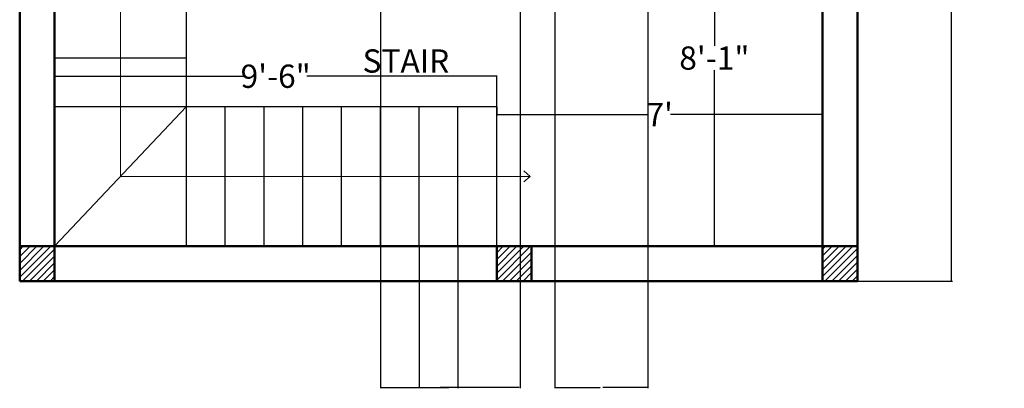
# Model space of a CAD drawing. Units: inches. Extents: x 0 to 281, y -535 to 46.
# Tile 1 of 22: x 27 to 281, y -535 to -440. Entities that reach past the tile are written whole.
import ezdxf

# ---------------------------------------------------------------- set-up
doc = ezdxf.new("R2010")
doc.units = ezdxf.units.IN
doc.header["$MEASUREMENT"] = 0
for name, color, linetype, lineweight in [('A-ANNO-DIMS', 2, 'Continuous', 18), ('A-ANNO-SYMB', 2, 'Continuous', 18), ('A-AREA-IDEN', 7, 'Continuous', 25), ('A-COLS', 7, 'Continuous', 50), ('A-COLS-PATT', 152, 'Continuous', 13), ('A-FLOR-STRS', 7, 'Continuous', 25), ('A-WALL', 7, 'Continuous', 50)]:
    doc.layers.add(name, color=color, linetype=linetype, lineweight=lineweight)
doc.styles.get("Standard").update_dxf_attribs({"font": 'arial.ttf'})
doc.dimstyles.get("Standard").update_dxf_attribs({"dimtxt": 0.18, "dimasz": 0.18, "dimexe": 0.18, "dimexo": 0.0625, "dimgap": 0.09, "dimtad": 0, "dimtih": 1, "dimtoh": 1, "dimdec": 0, "dimzin": 0, "dimdsep": 46, "dimlunit": 3, "dimtxsty": 'Standard', "dimcen": 0.09, "dimadec": 0, "dimazin": 0, "dimtfac": 1, "dimtdec": 0, "dimtofl": 0, "dimtmove": 0, "dimatfit": 3, "dimfxl": 1, "dimtolj": 1, "dimtzin": 0, "dimarcsym": 0})

# ---------------------------------------------------------------- blocks, each defined once
blk = doc.blocks.new('*D13')
at = {"layer": 'A-ANNO-DIMS', "color": 0, "lineweight": -2, "transparency": 16777216}
for p, q in [((206.57, -401.59), (206.57, -446.76)), ((206.63, -401.41), (206.75, -401.41)), ((206.57, -498.23), (206.57, -453.06)), ((206.63, -498.41), (206.75, -498.41))]:
    blk.add_line(p, q, dxfattribs=at)
at = {"layer": 'A-ANNO-DIMS', "color": 0, "transparency": 16777216}
for points in [[(206.54, -401.59), (206.6, -401.59), (206.57, -401.41)], [(206.54, -498.23), (206.6, -498.23), (206.57, -498.41)]]:
    blk.add_solid(points, dxfattribs=at)
at = {"layer": 'Defpoints', "color": 0, "transparency": 16777216}
for p in [(206.57, -401.41), (206.57, -498.41), (206.57, -498.41)]:
    blk.add_point(p, dxfattribs=at)
at = {"layer": 'A-ANNO-DIMS', "color": 0, "transparency": 16777216, "insert": (206.57, -449.91), "char_height": 6, "attachment_point": 5}
blk.add_mtext('\\A1;8\'-1"', dxfattribs=at)
blk = doc.blocks.new('*D14')
at = {"layer": 'A-ANNO-DIMS', "color": 0, "lineweight": -2, "transparency": 16777216}
for p, q in [((150.46, -462.47), (150.46, -464.67)), ((150.64, -464.49), (189.63, -464.49)), ((234.28, -464.49), (195.28, -464.49)), ((234.46, -462.47), (234.46, -464.67))]:
    blk.add_line(p, q, dxfattribs=at)
at = {"layer": 'A-ANNO-DIMS', "color": 0, "transparency": 16777216}
for points in [[(150.64, -464.46), (150.64, -464.52), (150.46, -464.49)], [(234.28, -464.46), (234.28, -464.52), (234.46, -464.49)]]:
    blk.add_solid(points, dxfattribs=at)
at = {"layer": 'Defpoints', "color": 0, "transparency": 16777216}
for p in [(150.46, -462.41), (234.46, -462.41), (234.46, -464.49)]:
    blk.add_point(p, dxfattribs=at)
at = {"layer": 'A-ANNO-DIMS', "color": 0, "transparency": 16777216, "insert": (192.46, -464.49), "char_height": 6, "attachment_point": 5}
blk.add_mtext("\\A1;7'", dxfattribs=at)
blk = doc.blocks.new('*D16')
at = {"layer": 'A-ANNO-DIMS', "color": 0, "lineweight": -2, "transparency": 16777216}
for p, q in [((36.46, -462.35), (36.46, -454.41)), ((150.46, -462.35), (150.46, -454.41)), ((36.64, -454.59), (85.39, -454.59)), ((150.28, -454.59), (101.52, -454.59))]:
    blk.add_line(p, q, dxfattribs=at)
at = {"layer": 'A-ANNO-DIMS', "color": 0, "transparency": 16777216}
for points in [[(36.64, -454.56), (36.64, -454.62), (36.46, -454.59)], [(150.28, -454.56), (150.28, -454.62), (150.46, -454.59)]]:
    blk.add_solid(points, dxfattribs=at)
at = {"layer": 'Defpoints', "color": 0, "transparency": 16777216}
for p in [(36.46, -454.59), (36.46, -462.41), (150.46, -462.41)]:
    blk.add_point(p, dxfattribs=at)
at = {"layer": 'A-ANNO-DIMS', "color": 0, "transparency": 16777216, "insert": (93.46, -454.59), "char_height": 6, "attachment_point": 5}
blk.add_mtext('\\A1;9\'-6"', dxfattribs=at)
blk = doc.blocks.new('*D18')
at = {"layer": 'A-ANNO-DIMS', "color": 0, "lineweight": -2, "transparency": 16777216}
for p, q in [((243.52, 18.59), (267.93, 18.59)), ((267.75, 18.41), (267.75, -241.26)), ((267.75, -507.23), (267.75, -247.57)), ((243.52, -507.41), (267.93, -507.41))]:
    blk.add_line(p, q, dxfattribs=at)
at = {"layer": 'A-ANNO-DIMS', "color": 0, "transparency": 16777216}
for points in [[(267.72, 18.41), (267.78, 18.41), (267.75, 18.59)], [(267.72, -507.23), (267.78, -507.23), (267.75, -507.41)]]:
    blk.add_solid(points, dxfattribs=at)
at = {"layer": 'Defpoints', "color": 0, "transparency": 16777216}
for p in [(243.46, 18.59), (243.46, -507.41), (267.75, -507.41)]:
    blk.add_point(p, dxfattribs=at)
at = {"layer": 'A-ANNO-DIMS', "color": 0, "transparency": 16777216, "insert": (267.75, -244.41), "char_height": 6, "attachment_point": 5}
blk.add_mtext('\\A1;43\'-10"', dxfattribs=at)
blk = doc.blocks.new('*D41')
at = {"layer": 'A-ANNO-DIMS', "color": 0, "lineweight": -2, "transparency": 16777216}
for p, q in [((120.46, -131.47), (120.46, -535.04)), ((156.46, -131.47), (156.46, -535.04)), ((120.64, -534.86), (138.13, -534.86)), ((156.28, -534.86), (138.79, -534.86))]:
    blk.add_line(p, q, dxfattribs=at)
at = {"layer": 'A-ANNO-DIMS', "color": 0, "transparency": 16777216}
for points in [[(120.64, -534.83), (120.64, -534.89), (120.46, -534.86)], [(156.28, -534.83), (156.28, -534.89), (156.46, -534.86)]]:
    blk.add_solid(points, dxfattribs=at)
at = {"layer": 'Defpoints', "color": 0, "transparency": 16777216}
for p in [(120.46, -131.41), (156.46, -131.41), (156.46, -534.86)]:
    blk.add_point(p, dxfattribs=at)
at = {"layer": 'A-ANNO-DIMS', "color": 0, "transparency": 16777216, "insert": (138.46, -534.86), "char_height": 0.18, "attachment_point": 5}
blk.add_mtext('\\A1;3\'-0"', dxfattribs=at)
blk = doc.blocks.new('*D42')
at = {"layer": 'A-ANNO-DIMS', "color": 0, "lineweight": -2, "transparency": 16777216}
for p, q in [((165.46, -131.47), (165.46, -535.04)), ((189.46, -131.47), (189.46, -535.04)), ((165.64, -534.86), (177.13, -534.86)), ((189.28, -534.86), (177.79, -534.86))]:
    blk.add_line(p, q, dxfattribs=at)
at = {"layer": 'A-ANNO-DIMS', "color": 0, "transparency": 16777216}
for points in [[(165.64, -534.83), (165.64, -534.89), (165.46, -534.86)], [(189.28, -534.83), (189.28, -534.89), (189.46, -534.86)]]:
    blk.add_solid(points, dxfattribs=at)
at = {"layer": 'Defpoints', "color": 0, "transparency": 16777216}
for p in [(165.46, -131.41), (189.46, -131.41), (189.46, -534.86)]:
    blk.add_point(p, dxfattribs=at)
at = {"layer": 'A-ANNO-DIMS', "color": 0, "transparency": 16777216, "insert": (177.46, -534.86), "char_height": 0.18, "attachment_point": 5}
blk.add_mtext('\\A1;2\'-0"', dxfattribs=at)
blk = doc.blocks.new('*D49')
at = {"layer": 'A-ANNO-DIMS', "color": 0, "lineweight": -2, "transparency": 16777216}
for p, q in [((130.46, -498.47), (130.46, -535.04)), ((140.46, -498.47), (140.46, -535.04)), ((130.64, -534.86), (135.06, -534.86)), ((140.28, -534.86), (135.86, -534.86))]:
    blk.add_line(p, q, dxfattribs=at)
at = {"layer": 'A-ANNO-DIMS', "color": 0, "transparency": 16777216}
for points in [[(130.64, -534.83), (130.64, -534.89), (130.46, -534.86)], [(140.28, -534.83), (140.28, -534.89), (140.46, -534.86)]]:
    blk.add_solid(points, dxfattribs=at)
at = {"layer": 'Defpoints', "color": 0, "transparency": 16777216}
for p in [(130.46, -498.41), (140.46, -498.41), (140.46, -534.86)]:
    blk.add_point(p, dxfattribs=at)
at = {"layer": 'A-ANNO-DIMS', "color": 0, "transparency": 16777216, "insert": (135.46, -534.86), "char_height": 0.18, "attachment_point": 5}
blk.add_mtext('\\A1;0\'-10"', dxfattribs=at)

msp = doc.modelspace()

# ---------------------------------------------------------------- hatches: boundary and pattern name
at = {"layer": 'A-COLS-PATT'}
h = msp.add_hatch(dxfattribs=at)
h.set_pattern_fill('ANSI31', color=256, scale=10)
h.paths.add_polyline_path([(36.46, 18.59), (27.46, 18.59), (27.46, 9.59), (36.46, 9.59)])
h.paths.add_polyline_path([(165.46, 18.59), (156.46, 18.59), (156.46, 9.59), (165.46, 9.59)])
h.paths.add_polyline_path([(243.46, 18.59), (234.46, 18.59), (234.46, 9.59), (243.46, 9.59)])
h.paths.add_polyline_path([(243.46, -122.41), (234.46, -122.41), (234.46, -131.41), (243.46, -131.41)])
h.paths.add_polyline_path([(36.46, -122.41), (27.46, -122.41), (27.46, -131.41), (36.46, -131.41)])
h.paths.add_polyline_path([(36.46, -498.41), (27.46, -498.41), (27.46, -507.41), (36.46, -507.41)])
h.paths.add_polyline_path([(243.46, -498.41), (234.46, -498.41), (234.46, -507.41), (243.46, -507.41)])
h.paths.add_polyline_path([(159.46, -498.41), (150.46, -498.41), (150.46, -507.41), (159.46, -507.41)])
h.paths.add_polyline_path([(36.46, -392.41), (27.46, -392.41), (27.46, -401.41), (36.46, -401.41)])
h.paths.add_polyline_path([(159.46, -392.41), (150.46, -392.41), (150.46, -401.41), (159.46, -401.41)])
h.paths.add_polyline_path([(243.46, -392.41), (234.46, -392.41), (234.46, -401.41), (243.46, -401.41)])
h.paths.add_polyline_path([(36.46, -263.41), (27.46, -263.41), (27.46, -272.41), (36.46, -272.41)])
h.paths.add_polyline_path([(243.46, -263.41), (234.46, -263.41), (234.46, -272.41), (243.46, -272.41)])

# ---------------------------------------------------------------- linework, layer by layer
at = {"layer": 'A-ANNO-SYMB'}
for p, q in [((53.46, -419.41), (53.46, -480.41)), ((159.11, -480.41), (157.42, -479)), ((53.46, -480.41), (159.11, -480.41)), ((159.11, -480.41), (157.42, -481.82))]:
    msp.add_line(p, q, dxfattribs=at)
at = {"layer": 'A-COLS'}
for p, q in [((150.46, -498.41), (150.46, -507.41)), ((159.46, -498.41), (159.46, -507.41))]:
    msp.add_line(p, q, dxfattribs=at)
at = {"layer": 'A-FLOR-STRS'}
for p, q in [((70.46, -498.41), (70.46, -401.41)), ((70.46, -449.91), (36.46, -449.91)), ((36.46, -462.41), (150.46, -462.41)), ((70.46, -462.41), (36.46, -498.41)), ((80.46, -498.41), (80.46, -462.41)), ((90.46, -498.41), (90.46, -462.41)), ((100.46, -498.41), (100.46, -462.41)), ((110.46, -498.41), (110.46, -462.41)), ((120.46, -498.41), (120.46, -462.41)), ((130.46, -498.41), (130.46, -462.41)), ((140.46, -498.41), (140.46, -462.41)), ((150.46, -498.41), (150.46, -462.41))]:
    msp.add_line(p, q, dxfattribs=at)
at = {"layer": 'A-WALL'}
for p, q in [((27.46, 18.59), (27.46, -507.41)), ((36.46, 18.59), (36.46, -507.41)), ((234.46, 18.59), (234.46, -507.41)), ((243.46, 18.59), (243.46, -507.41)), ((27.46, -498.41), (243.46, -498.41)), ((27.46, -507.41), (243.46, -507.41))]:
    msp.add_line(p, q, dxfattribs=at)

# ---------------------------------------------------------------- texts
at = {"layer": 'A-AREA-IDEN', "insert": (115.86, -447.66), "char_height": 6, "attachment_point": 1}
msp.add_mtext('STAIR', dxfattribs=at)

# ---------------------------------------------------------------- dimensions: what is measured, and where the dimension line sits
at = {"layer": 'A-ANNO-DIMS'}
for base, p1, p2, picture, middle in [((267.75, -507.41), (243.46, 18.59), (243.46, -507.41), '*D18', (267.75, -244.41)), ((206.57, -498.41), (206.57, -401.41), (206.57, -498.41), '*D13', (206.57, -449.91))]:
    dim = msp.add_linear_dim(base=base, p1=p1, p2=p2, angle=90, dimstyle='Standard', override={"dimtxt": 6, "dimclrd": 0, "dimclre": 0, "dimclrt": 0}, dxfattribs=at)
    dim.commit()
    dim.dimension.update_dxf_attribs({"geometry": picture, "text_midpoint": middle})
for base, p1, p2, override, picture, middle in [((156.46, -534.86), (120.46, -131.41), (156.46, -131.41), {"dimdec": 1, "dimlfac": 1, "dimrnd": 0, "dimzin": 1, "dimdsep": 46, "dimlunit": 4, "dimfrac": 2}, '*D41', (138.46, -534.86)), ((189.46, -534.86), (165.46, -131.41), (189.46, -131.41), {"dimdec": 1, "dimlfac": 1, "dimrnd": 0, "dimzin": 1, "dimdsep": 46, "dimlunit": 4, "dimfrac": 2}, '*D42', (177.46, -534.86)), ((36.46, -454.59), (150.46, -462.41), (36.46, -462.41), {"dimtxt": 6, "dimclrd": 0, "dimclre": 0, "dimclrt": 0}, '*D16', (93.46, -454.59)), ((234.46, -464.49), (150.46, -462.41), (234.46, -462.41), {"dimtxt": 6, "dimclrd": 0, "dimclre": 0, "dimclrt": 0}, '*D14', (192.46, -464.49)), ((140.46, -534.86), (130.46, -498.41), (140.46, -498.41), {"dimdec": 1, "dimlfac": 1, "dimrnd": 0, "dimzin": 1, "dimdsep": 46, "dimlunit": 4, "dimfrac": 2}, '*D49', (135.46, -534.86))]:
    dim = msp.add_linear_dim(base=base, p1=p1, p2=p2, dimstyle='Standard', override=override, dxfattribs=at)
    dim.commit()
    dim.dimension.update_dxf_attribs({"geometry": picture, "text_midpoint": middle})

doc.saveas('drawing.dxf')
